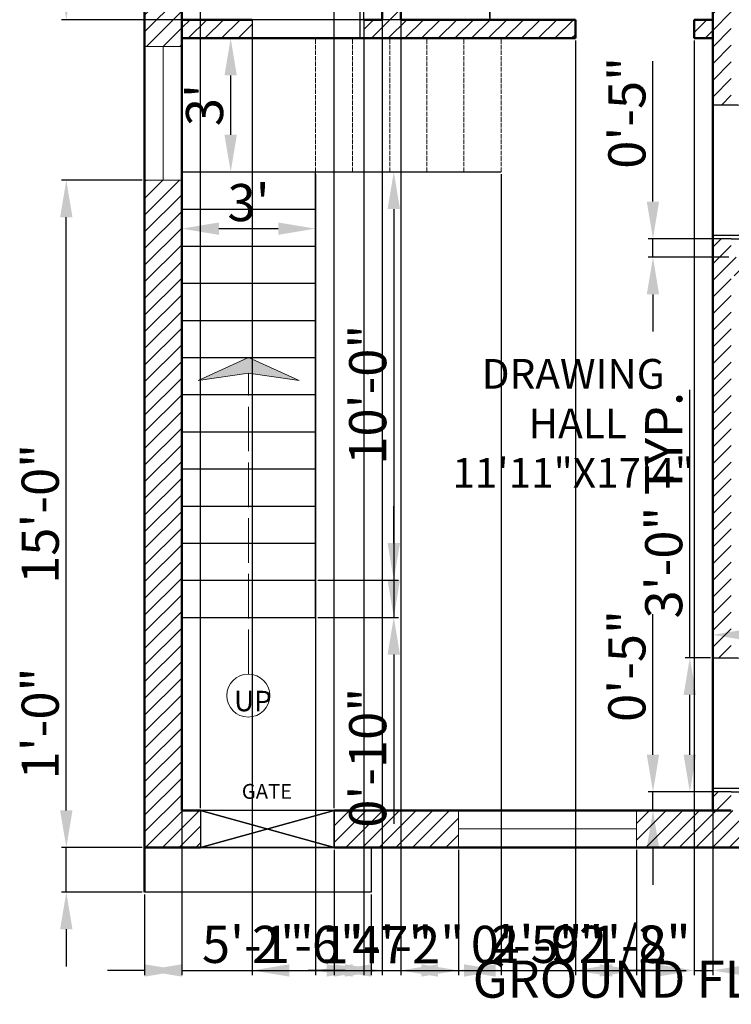
# Model space of a CAD drawing. Units: inches. Extents: x 2305 to 2787, y 1816 to 2216.
# Tile 1 of 3: x 2305 to 2496, y 1816 to 2081. Entities that reach past the tile are written whole.
import ezdxf

# ---------------------------------------------------------------- set-up
doc = ezdxf.new("R2010")
doc.units = ezdxf.units.IN
doc.linetypes.add('ACAD_ISO02W100', pattern=[15, 12, -3])
for name, color, linetype, lineweight in [('A-ANNO-DIMS', 2, 'Continuous', 18), ('A-ANNO-PATH', 253, 'ACAD_ISO02W100', 18), ('A-ANNO-SYMB', 253, 'Continuous', 18), ('A-ANNO-TEXT', 7, 'Continuous', 25), ('A-AREA-IDEN', 7, 'Continuous', 25), ('A-DOOR', 4, 'Continuous', 25), ('A-DOOR-GATE', 240, 'Continuous', 25), ('A-FLOR-FIXT', 8, 'Continuous', 25), ('A-FLOR-STRS', 7, 'Continuous', 25), ('A-FLOR-STRS-OVHD', 253, 'ACAD_ISO02W100', 18), ('A-GLAZ', 4, 'Continuous', 18), ('A-WALL', 7, 'Continuous', 50), ('A-WALL-PATT', 8, 'Continuous', 13)]:
    doc.layers.add(name, color=color, linetype=linetype, lineweight=lineweight)
doc.styles.get("Standard").update_dxf_attribs({"font": 'arial.ttf'})
doc.dimstyles.new('ISO-25', dxfattribs={"dimtxt": 10, "dimasz": 10, "dimexe": 1.25, "dimexo": 0.625, "dimtad": 1, "dimdec": 1, "dimlunit": 3, "dimtxsty": 'Standard', "dimcen": 2.5, "dimadec": 0, "dimazin": 0, "dimtfac": 1, "dimtdec": 1, "dimtmove": 0, "dimatfit": 3, "dimfxl": 1, "dimarcsym": 0})

# ---------------------------------------------------------------- blocks, each defined once
blk = doc.blocks.new('*D7')
at = {"layer": 'A-ANNO-DIMS', "color": 0, "lineweight": -2, "transparency": 16777216}
for p, q in [((2348.79, 2076), (2362.59, 2076)), ((2361.34, 2050), (2361.34, 2066)), ((2348.79, 2040), (2362.59, 2040))]:
    blk.add_line(p, q, dxfattribs=at)
at = {"layer": 'A-ANNO-DIMS', "color": 0, "transparency": 16777216}
for points in [[(2359.67, 2066), (2363, 2066), (2361.34, 2076)], [(2359.67, 2050), (2363, 2050), (2361.34, 2040)]]:
    blk.add_solid(points, dxfattribs=at)
at = {"layer": 'Defpoints', "color": 0, "transparency": 16777216}
for p in [(2348.17, 2076), (2361.34, 2076), (2348.17, 2040)]:
    blk.add_point(p, dxfattribs=at)
at = {"layer": 'A-ANNO-DIMS', "color": 0, "transparency": 16777216, "insert": (2355.6, 2058), "char_height": 10, "attachment_point": 5, "rotation": 90}
blk.add_mtext("3'", dxfattribs=at)
blk = doc.blocks.new('*D8')
at = {"layer": 'A-ANNO-DIMS', "color": 0, "lineweight": -2, "transparency": 16777216}
for p, q in [((2348.17, 2029.37), (2348.17, 2023.46)), ((2384.17, 2029.37), (2384.17, 2023.46)), ((2358.17, 2024.71), (2374.17, 2024.71))]:
    blk.add_line(p, q, dxfattribs=at)
at = {"layer": 'A-ANNO-DIMS', "color": 0, "transparency": 16777216}
for points in [[(2358.17, 2026.37), (2358.17, 2023.04), (2348.17, 2024.71)], [(2374.17, 2026.37), (2374.17, 2023.04), (2384.17, 2024.71)]]:
    blk.add_solid(points, dxfattribs=at)
at = {"layer": 'Defpoints', "color": 0, "transparency": 16777216}
for p in [(2348.17, 2030), (2384.17, 2030), (2384.17, 2024.71)]:
    blk.add_point(p, dxfattribs=at)
at = {"layer": 'A-ANNO-DIMS', "color": 0, "transparency": 16777216, "insert": (2366.17, 2030.44), "char_height": 10, "attachment_point": 5}
blk.add_mtext("3'", dxfattribs=at)
blk = doc.blocks.new('DOOR-SWING-36IN')
for p, q in [((5, 36), (0, 36)), ((0, 1), (41, 1)), ((5, 0), (0, 0)), ((5, 0), (41, 0))]:
    blk.add_line(p, q)
blk.add_arc((5.5, 0.5), 35.5, 359.1931, 90.8069)
blk = doc.blocks.new('WINDOW-36IN')
for p, q in [((0, 10), (0, 0)), ((36, 10), (36, 0)), ((0, 5), (36, 5))]:
    blk.add_line(p, q)
blk = doc.blocks.new('*D18')
at = {"layer": 'A-ANNO-DIMS', "color": 0, "lineweight": -2, "transparency": 16777216}
for p, q in [((2491.17, 1909.76), (2491.17, 1916.55)), ((2501.17, 1915.3), (2522.3, 1915.3)), ((2532.3, 1909.76), (2532.3, 1916.55)), ((2532.3, 1915.3), (2649.8, 1915.3))]:
    blk.add_line(p, q, dxfattribs=at)
at = {"layer": 'A-ANNO-DIMS', "color": 0, "transparency": 16777216}
for points in [[(2501.17, 1916.97), (2501.17, 1913.63), (2491.17, 1915.3)], [(2522.3, 1916.97), (2522.3, 1913.63), (2532.3, 1915.3)]]:
    blk.add_solid(points, dxfattribs=at)
at = {"layer": 'Defpoints', "color": 0, "transparency": 16777216}
for p in [(2532.3, 1915.3), (2491.17, 1909.13), (2532.3, 1909.13)]:
    blk.add_point(p, dxfattribs=at)
at = {"layer": 'A-ANNO-DIMS', "color": 0, "transparency": 16777216, "insert": (2596.05, 1921.1), "char_height": 10, "attachment_point": 5}
blk.add_mtext('DOOR 3\'-5" TYP.', dxfattribs=at)
blk = doc.blocks.new('*D19')
at = {"layer": 'A-ANNO-DIMS', "color": 0, "lineweight": -2, "transparency": 16777216}
for p, q in [((2485, 1909.13), (2485, 1981.33)), ((2490.54, 1909.13), (2483.75, 1909.13)), ((2485, 1883), (2485, 1899.13)), ((2490.54, 1873), (2483.75, 1873))]:
    blk.add_line(p, q, dxfattribs=at)
at = {"layer": 'A-ANNO-DIMS', "color": 0, "transparency": 16777216}
for points in [[(2483.33, 1899.13), (2486.66, 1899.13), (2485, 1909.13)], [(2483.33, 1883), (2486.66, 1883), (2485, 1873)]]:
    blk.add_solid(points, dxfattribs=at)
at = {"layer": 'Defpoints', "color": 0, "transparency": 16777216}
for p in [(2485, 1909.13), (2491.17, 1909.13), (2491.17, 1873)]:
    blk.add_point(p, dxfattribs=at)
at = {"layer": 'A-ANNO-DIMS', "color": 0, "transparency": 16777216, "insert": (2479.26, 1950.23), "char_height": 10, "attachment_point": 5, "rotation": 90}
blk.add_mtext('3\'-0" TYP.', dxfattribs=at)
blk = doc.blocks.new('*D29')
at = {"layer": 'A-ANNO-DIMS', "color": 0, "lineweight": -2, "transparency": 16777216}
for p, q in [((2348.17, 1868.62), (2348.17, 2180.35)), ((2353.17, 1868.62), (2353.17, 2180.35)), ((2338.17, 2179.1), (2328.17, 2179.1)), ((2348.17, 2179.1), (2353.17, 2179.1)), ((2363.17, 2179.1), (2401, 2179.1))]:
    blk.add_line(p, q, dxfattribs=at)
at = {"layer": 'A-ANNO-DIMS', "color": 0, "transparency": 16777216}
for points in [[(2338.17, 2180.76), (2338.17, 2177.43), (2348.17, 2179.1)], [(2363.17, 2180.76), (2363.17, 2177.43), (2353.17, 2179.1)]]:
    blk.add_solid(points, dxfattribs=at)
at = {"layer": 'Defpoints', "color": 0, "transparency": 16777216}
for p in [(2353.17, 2179.1), (2348.17, 1868), (2353.17, 1868)]:
    blk.add_point(p, dxfattribs=at)
at = {"layer": 'A-ANNO-DIMS', "color": 0, "transparency": 16777216, "insert": (2387.08, 2184.83), "char_height": 10, "attachment_point": 5}
blk.add_mtext('0\'-5"', dxfattribs=at)
blk = doc.blocks.new('*D30')
at = {"layer": 'A-ANNO-DIMS', "color": 0, "lineweight": -2, "transparency": 16777216}
for p, q in [((2353.17, 1868.62), (2353.17, 2180.35)), ((2389.17, 1868.62), (2389.17, 2180.35)), ((2363.17, 2179.1), (2379.17, 2179.1))]:
    blk.add_line(p, q, dxfattribs=at)
at = {"layer": 'A-ANNO-DIMS', "color": 0, "transparency": 16777216}
for points in [[(2363.17, 2180.76), (2363.17, 2177.43), (2353.17, 2179.1)], [(2379.17, 2180.76), (2379.17, 2177.43), (2389.17, 2179.1)]]:
    blk.add_solid(points, dxfattribs=at)
at = {"layer": 'Defpoints', "color": 0, "transparency": 16777216}
for p in [(2389.17, 2179.1), (2353.17, 1868), (2389.17, 1868)]:
    blk.add_point(p, dxfattribs=at)
at = {"layer": 'A-ANNO-DIMS', "color": 0, "transparency": 16777216, "insert": (2371.17, 2184.83), "char_height": 10, "attachment_point": 5}
blk.add_mtext('3\'-0"', dxfattribs=at)
blk = doc.blocks.new('*D31')
at = {"layer": 'A-ANNO-DIMS', "color": 0, "lineweight": -2, "transparency": 16777216}
for p, q in [((2389.17, 1857.37), (2389.17, 1823.65)), ((2422.67, 1857.37), (2422.67, 1823.65)), ((2399.17, 1824.9), (2412.67, 1824.9)), ((2422.67, 1824.9), (2483.97, 1824.9))]:
    blk.add_line(p, q, dxfattribs=at)
at = {"layer": 'A-ANNO-DIMS', "color": 0, "transparency": 16777216}
for points in [[(2399.17, 1826.56), (2399.17, 1823.23), (2389.17, 1824.9)], [(2412.67, 1826.56), (2412.67, 1823.23), (2422.67, 1824.9)]]:
    blk.add_solid(points, dxfattribs=at)
at = {"layer": 'Defpoints', "color": 0, "transparency": 16777216}
for p in [(2389.17, 1858), (2422.67, 1858), (2422.67, 1824.9)]:
    blk.add_point(p, dxfattribs=at)
at = {"layer": 'A-ANNO-DIMS', "color": 0, "transparency": 16777216, "insert": (2458.32, 1830.69), "char_height": 10, "attachment_point": 5}
blk.add_mtext('2\'-9 1/2"', dxfattribs=at)
blk = doc.blocks.new('*D32')
at = {"layer": 'A-ANNO-DIMS', "color": 0, "lineweight": -2, "transparency": 16777216}
for p, q in [((2422.67, 1857.37), (2422.67, 1823.65)), ((2470.67, 1857.37), (2470.67, 1823.65)), ((2432.67, 1824.9), (2460.67, 1824.9))]:
    blk.add_line(p, q, dxfattribs=at)
at = {"layer": 'A-ANNO-DIMS', "color": 0, "transparency": 16777216}
for points in [[(2432.67, 1826.56), (2432.67, 1823.23), (2422.67, 1824.9)], [(2460.67, 1826.56), (2460.67, 1823.23), (2470.67, 1824.9)]]:
    blk.add_solid(points, dxfattribs=at)
at = {"layer": 'Defpoints', "color": 0, "transparency": 16777216}
for p in [(2422.67, 1858), (2470.67, 1858), (2470.67, 1824.9)]:
    blk.add_point(p, dxfattribs=at)
at = {"layer": 'A-ANNO-DIMS', "color": 0, "transparency": 16777216, "insert": (2446.67, 1830.63), "char_height": 10, "attachment_point": 5}
blk.add_mtext('4\'-0"', dxfattribs=at)
blk = doc.blocks.new('*D34')
at = {"layer": 'A-ANNO-DIMS', "color": 0, "lineweight": -2, "transparency": 16777216}
for p, q in [((2337.54, 2037.78), (2315.82, 2037.78)), ((2317.07, 1868), (2317.07, 2027.78)), ((2337.54, 1858), (2315.82, 1858))]:
    blk.add_line(p, q, dxfattribs=at)
at = {"layer": 'A-ANNO-DIMS', "color": 0, "transparency": 16777216}
for points in [[(2315.4, 2027.78), (2318.73, 2027.78), (2317.07, 2037.78)], [(2315.4, 1868), (2318.73, 1868), (2317.07, 1858)]]:
    blk.add_solid(points, dxfattribs=at)
at = {"layer": 'Defpoints', "color": 0, "transparency": 16777216}
for p in [(2317.07, 2037.78), (2338.17, 2037.78), (2338.17, 1858)]:
    blk.add_point(p, dxfattribs=at)
at = {"layer": 'A-ANNO-DIMS', "color": 0, "transparency": 16777216, "insert": (2311.34, 1947.89), "char_height": 10, "attachment_point": 5, "rotation": 90}
blk.add_mtext('15\'-0"', dxfattribs=at)
blk = doc.blocks.new('*D35')
at = {"layer": 'A-ANNO-DIMS', "color": 0, "lineweight": -2, "transparency": 16777216}
for p, q in [((2338.17, 1845.37), (2338.17, 1823.65)), ((2399.17, 1845.37), (2399.17, 1823.65)), ((2348.17, 1824.9), (2389.17, 1824.9))]:
    blk.add_line(p, q, dxfattribs=at)
at = {"layer": 'A-ANNO-DIMS', "color": 0, "transparency": 16777216}
for points in [[(2348.17, 1826.56), (2348.17, 1823.23), (2338.17, 1824.9)], [(2389.17, 1826.56), (2389.17, 1823.23), (2399.17, 1824.9)]]:
    blk.add_solid(points, dxfattribs=at)
at = {"layer": 'Defpoints', "color": 0, "transparency": 16777216}
for p in [(2338.17, 1846), (2399.17, 1846), (2399.17, 1824.9)]:
    blk.add_point(p, dxfattribs=at)
at = {"layer": 'A-ANNO-DIMS', "color": 0, "transparency": 16777216, "insert": (2368.67, 1830.63), "char_height": 10, "attachment_point": 5}
blk.add_mtext('5\'-1"', dxfattribs=at)
blk = doc.blocks.new('*D36')
at = {"layer": 'A-ANNO-DIMS', "color": 0, "lineweight": -2, "transparency": 16777216}
for p, q in [((2317.07, 1868), (2317.07, 1904.89)), ((2337.54, 1858), (2315.82, 1858)), ((2317.07, 1846), (2317.07, 1858)), ((2337.54, 1846), (2315.82, 1846)), ((2317.07, 1836), (2317.07, 1826))]:
    blk.add_line(p, q, dxfattribs=at)
at = {"layer": 'A-ANNO-DIMS', "color": 0, "transparency": 16777216}
for points in [[(2315.4, 1868), (2318.73, 1868), (2317.07, 1858)], [(2315.4, 1836), (2318.73, 1836), (2317.07, 1846)]]:
    blk.add_solid(points, dxfattribs=at)
at = {"layer": 'Defpoints', "color": 0, "transparency": 16777216}
for p in [(2317.07, 1858), (2338.17, 1858), (2338.17, 1846)]:
    blk.add_point(p, dxfattribs=at)
at = {"layer": 'A-ANNO-DIMS', "color": 0, "transparency": 16777216, "insert": (2311.34, 1891.44), "char_height": 10, "attachment_point": 5, "rotation": 90}
blk.add_mtext('1\'-0"', dxfattribs=at)
blk = doc.blocks.new('*D37')
at = {"layer": 'A-ANNO-DIMS', "color": 0, "lineweight": -2, "transparency": 16777216}
for p, q in [((2367.17, 2080.37), (2367.17, 1823.65)), ((2397.17, 2080.37), (2397.17, 1823.65)), ((2377.17, 1824.9), (2387.17, 1824.9))]:
    blk.add_line(p, q, dxfattribs=at)
at = {"layer": 'A-ANNO-DIMS', "color": 0, "transparency": 16777216}
for points in [[(2377.17, 1826.56), (2377.17, 1823.23), (2367.17, 1824.9)], [(2387.17, 1826.56), (2387.17, 1823.23), (2397.17, 1824.9)]]:
    blk.add_solid(points, dxfattribs=at)
at = {"layer": 'Defpoints', "color": 0, "transparency": 16777216}
for p in [(2367.17, 2081), (2397.17, 2081), (2397.17, 1824.9)]:
    blk.add_point(p, dxfattribs=at)
at = {"layer": 'A-ANNO-DIMS', "color": 0, "transparency": 16777216, "insert": (2382.17, 1830.63), "char_height": 10, "attachment_point": 5}
blk.add_mtext('2\'-6"', dxfattribs=at)
blk = doc.blocks.new('*D38')
at = {"layer": 'A-ANNO-DIMS', "color": 0, "lineweight": -2, "transparency": 16777216}
for p, q in [((2454.17, 2075.37), (2454.17, 1823.65)), ((2486.17, 2075.37), (2486.17, 1823.65)), ((2464.17, 1824.9), (2476.17, 1824.9))]:
    blk.add_line(p, q, dxfattribs=at)
at = {"layer": 'A-ANNO-DIMS', "color": 0, "transparency": 16777216}
for points in [[(2464.17, 1826.56), (2464.17, 1823.23), (2454.17, 1824.9)], [(2476.17, 1826.56), (2476.17, 1823.23), (2486.17, 1824.9)]]:
    blk.add_solid(points, dxfattribs=at)
at = {"layer": 'Defpoints', "color": 0, "transparency": 16777216}
for p in [(2454.17, 2076), (2486.17, 2076), (2486.17, 1824.9)]:
    blk.add_point(p, dxfattribs=at)
at = {"layer": 'A-ANNO-DIMS', "color": 0, "transparency": 16777216, "insert": (2470.17, 1830.63), "char_height": 10, "attachment_point": 5}
blk.add_mtext('2\'-8"', dxfattribs=at)
blk = doc.blocks.new('*D39')
at = {"layer": 'A-ANNO-DIMS', "color": 0, "lineweight": -2, "transparency": 16777216}
for p, q in [((2402.17, 2147.37), (2402.17, 1823.65)), ((2407.17, 2147.37), (2407.17, 1823.65)), ((2392.17, 1824.9), (2382.17, 1824.9)), ((2402.17, 1824.9), (2407.17, 1824.9)), ((2417.17, 1824.9), (2455, 1824.9))]:
    blk.add_line(p, q, dxfattribs=at)
at = {"layer": 'A-ANNO-DIMS', "color": 0, "transparency": 16777216}
for points in [[(2392.17, 1826.56), (2392.17, 1823.23), (2402.17, 1824.9)], [(2417.17, 1826.56), (2417.17, 1823.23), (2407.17, 1824.9)]]:
    blk.add_solid(points, dxfattribs=at)
at = {"layer": 'Defpoints', "color": 0, "transparency": 16777216}
for p in [(2402.17, 2148), (2407.17, 2148), (2407.17, 1824.9)]:
    blk.add_point(p, dxfattribs=at)
at = {"layer": 'A-ANNO-DIMS', "color": 0, "transparency": 16777216, "insert": (2441.08, 1830.63), "char_height": 10, "attachment_point": 5}
blk.add_mtext('0\'-5"', dxfattribs=at)
blk = doc.blocks.new('*D40')
at = {"layer": 'A-ANNO-DIMS', "color": 0, "lineweight": -2, "transparency": 16777216}
for p, q in [((2384.79, 2040), (2406.52, 2040)), ((2405.27, 2030), (2405.27, 1930)), ((2384.79, 1920), (2406.52, 1920))]:
    blk.add_line(p, q, dxfattribs=at)
at = {"layer": 'A-ANNO-DIMS', "color": 0, "transparency": 16777216}
for points in [[(2403.6, 2030), (2406.93, 2030), (2405.27, 2040)], [(2403.6, 1930), (2406.93, 1930), (2405.27, 1920)]]:
    blk.add_solid(points, dxfattribs=at)
at = {"layer": 'Defpoints', "color": 0, "transparency": 16777216}
for p in [(2384.17, 2040), (2384.17, 1920), (2405.27, 1920)]:
    blk.add_point(p, dxfattribs=at)
at = {"layer": 'A-ANNO-DIMS', "color": 0, "transparency": 16777216, "insert": (2399.54, 1980), "char_height": 10, "attachment_point": 5, "rotation": 90}
blk.add_mtext('10\'-0"', dxfattribs=at)
blk = doc.blocks.new('*D41')
at = {"layer": 'A-ANNO-DIMS', "color": 0, "lineweight": -2, "transparency": 16777216}
for p, q in [((2405.27, 1940), (2405.27, 1950)), ((2384.79, 1930), (2406.52, 1930)), ((2405.27, 1930), (2405.27, 1920)), ((2384.79, 1920), (2406.52, 1920)), ((2405.27, 1910), (2405.27, 1864.39))]:
    blk.add_line(p, q, dxfattribs=at)
at = {"layer": 'A-ANNO-DIMS', "color": 0, "transparency": 16777216}
for points in [[(2403.6, 1940), (2406.93, 1940), (2405.27, 1930)], [(2403.6, 1910), (2406.93, 1910), (2405.27, 1920)]]:
    blk.add_solid(points, dxfattribs=at)
at = {"layer": 'Defpoints', "color": 0, "transparency": 16777216}
for p in [(2384.17, 1930), (2384.17, 1920), (2405.27, 1920)]:
    blk.add_point(p, dxfattribs=at)
at = {"layer": 'A-ANNO-DIMS', "color": 0, "transparency": 16777216, "insert": (2399.54, 1882.19), "char_height": 10, "attachment_point": 5, "rotation": 90}
blk.add_mtext('0\'-10"', dxfattribs=at)
blk = doc.blocks.new('*D42')
at = {"layer": 'A-ANNO-DIMS', "color": 0, "lineweight": -2, "transparency": 16777216}
for p, q in [((2384.17, 2039.37), (2384.17, 1823.65)), ((2434.17, 2039.37), (2434.17, 1823.65)), ((2394.17, 1824.9), (2424.17, 1824.9))]:
    blk.add_line(p, q, dxfattribs=at)
at = {"layer": 'A-ANNO-DIMS', "color": 0, "transparency": 16777216}
for points in [[(2394.17, 1826.56), (2394.17, 1823.23), (2384.17, 1824.9)], [(2424.17, 1826.56), (2424.17, 1823.23), (2434.17, 1824.9)]]:
    blk.add_solid(points, dxfattribs=at)
at = {"layer": 'Defpoints', "color": 0, "transparency": 16777216}
for p in [(2384.17, 2040), (2434.17, 2040), (2434.17, 1824.9)]:
    blk.add_point(p, dxfattribs=at)
at = {"layer": 'A-ANNO-DIMS', "color": 0, "transparency": 16777216, "insert": (2409.17, 1830.54), "char_height": 10, "attachment_point": 5}
blk.add_mtext('4\'-2"', dxfattribs=at)
blk = doc.blocks.new('*D43')
at = {"layer": 'A-ANNO-DIMS', "color": 0, "lineweight": -2, "transparency": 16777216}
for p, q in [((2475.07, 2032), (2475.07, 2069.83)), ((2495.54, 2022), (2473.82, 2022)), ((2475.07, 2017), (2475.07, 2022)), ((2495.54, 2017), (2473.82, 2017)), ((2475.07, 2007), (2475.07, 1997))]:
    blk.add_line(p, q, dxfattribs=at)
at = {"layer": 'A-ANNO-DIMS', "color": 0, "transparency": 16777216}
for points in [[(2473.4, 2032), (2476.73, 2032), (2475.07, 2022)], [(2473.4, 2007), (2476.73, 2007), (2475.07, 2017)]]:
    blk.add_solid(points, dxfattribs=at)
at = {"layer": 'Defpoints', "color": 0, "transparency": 16777216}
for p in [(2475.07, 2022), (2496.17, 2022), (2496.17, 2017)]:
    blk.add_point(p, dxfattribs=at)
at = {"layer": 'A-ANNO-DIMS', "color": 0, "transparency": 16777216, "insert": (2469.34, 2055.91), "char_height": 10, "attachment_point": 5, "rotation": 90}
blk.add_mtext('0\'-5"', dxfattribs=at)
blk = doc.blocks.new('*D44')
at = {"layer": 'A-ANNO-DIMS', "color": 0, "lineweight": -2, "transparency": 16777216}
for p, q in [((2475.07, 1883), (2475.07, 1920.83)), ((2495.54, 1873), (2473.82, 1873)), ((2475.07, 1868), (2475.07, 1873)), ((2495.54, 1868), (2473.82, 1868)), ((2475.07, 1858), (2475.07, 1848))]:
    blk.add_line(p, q, dxfattribs=at)
at = {"layer": 'A-ANNO-DIMS', "color": 0, "transparency": 16777216}
for points in [[(2473.4, 1883), (2476.73, 1883), (2475.07, 1873)], [(2473.4, 1858), (2476.73, 1858), (2475.07, 1868)]]:
    blk.add_solid(points, dxfattribs=at)
at = {"layer": 'Defpoints', "color": 0, "transparency": 16777216}
for p in [(2475.07, 1873), (2496.17, 1873), (2496.17, 1868)]:
    blk.add_point(p, dxfattribs=at)
at = {"layer": 'A-ANNO-DIMS', "color": 0, "transparency": 16777216, "insert": (2469.34, 1906.91), "char_height": 10, "attachment_point": 5, "rotation": 90}
blk.add_mtext('0\'-5"', dxfattribs=at)
blk = doc.blocks.new('*D45')
at = {"layer": 'A-ANNO-DIMS', "color": 0, "lineweight": -2, "transparency": 16777216}
for p, q in [((2486.17, 2075.37), (2486.17, 1823.65)), ((2491.17, 2075.37), (2491.17, 1823.65)), ((2476.17, 1824.9), (2466.17, 1824.9)), ((2486.17, 1824.9), (2491.17, 1824.9)), ((2501.17, 1824.9), (2539, 1824.9))]:
    blk.add_line(p, q, dxfattribs=at)
at = {"layer": 'A-ANNO-DIMS', "color": 0, "transparency": 16777216}
for points in [[(2476.17, 1826.56), (2476.17, 1823.23), (2486.17, 1824.9)], [(2501.17, 1826.56), (2501.17, 1823.23), (2491.17, 1824.9)]]:
    blk.add_solid(points, dxfattribs=at)
at = {"layer": 'Defpoints', "color": 0, "transparency": 16777216}
for p in [(2486.17, 2076), (2491.17, 2076), (2491.17, 1824.9)]:
    blk.add_point(p, dxfattribs=at)
at = {"layer": 'A-ANNO-DIMS', "color": 0, "transparency": 16777216, "insert": (2525.08, 1830.63), "char_height": 10, "attachment_point": 5}
blk.add_mtext('0\'-5"', dxfattribs=at)
blk = doc.blocks.new('*D46')
at = {"layer": 'A-ANNO-DIMS', "color": 0, "lineweight": -2, "transparency": 16777216}
for p, q in [((2348.17, 2080.37), (2348.17, 1823.65)), ((2367.17, 2080.37), (2367.17, 1823.65)), ((2338.17, 1824.9), (2328.17, 1824.9)), ((2348.17, 1824.9), (2367.17, 1824.9)), ((2377.17, 1824.9), (2414.06, 1824.9))]:
    blk.add_line(p, q, dxfattribs=at)
at = {"layer": 'A-ANNO-DIMS', "color": 0, "transparency": 16777216}
for points in [[(2338.17, 1826.56), (2338.17, 1823.23), (2348.17, 1824.9)], [(2377.17, 1826.56), (2377.17, 1823.23), (2367.17, 1824.9)]]:
    blk.add_solid(points, dxfattribs=at)
at = {"layer": 'Defpoints', "color": 0, "transparency": 16777216}
for p in [(2348.17, 2081), (2367.17, 2081), (2367.17, 1824.9)]:
    blk.add_point(p, dxfattribs=at)
at = {"layer": 'A-ANNO-DIMS', "color": 0, "transparency": 16777216, "insert": (2400.61, 1830.54), "char_height": 10, "attachment_point": 5}
blk.add_mtext('1\'-7"', dxfattribs=at)
blk = doc.blocks.new('*D47')
at = {"layer": 'A-ANNO-DIMS', "color": 0, "lineweight": -2, "transparency": 16777216}
for p, q in [((2407.17, 2081.62), (2407.17, 2180.35)), ((2431.17, 2081.62), (2431.17, 2180.35)), ((2417.17, 2179.1), (2421.17, 2179.1)), ((2431.17, 2179.1), (2469.17, 2179.1))]:
    blk.add_line(p, q, dxfattribs=at)
at = {"layer": 'A-ANNO-DIMS', "color": 0, "transparency": 16777216}
for points in [[(2417.17, 2180.76), (2417.17, 2177.43), (2407.17, 2179.1)], [(2421.17, 2180.76), (2421.17, 2177.43), (2431.17, 2179.1)]]:
    blk.add_solid(points, dxfattribs=at)
at = {"layer": 'Defpoints', "color": 0, "transparency": 16777216}
for p in [(2431.17, 2179.1), (2407.17, 2081), (2431.17, 2081)]:
    blk.add_point(p, dxfattribs=at)
at = {"layer": 'A-ANNO-DIMS', "color": 0, "transparency": 16777216, "insert": (2455.17, 2184.83), "char_height": 10, "attachment_point": 5}
blk.add_mtext('2\'-0"', dxfattribs=at)
blk = doc.blocks.new('*D48')
at = {"layer": 'A-ANNO-DIMS', "color": 0, "lineweight": -2, "transparency": 16777216}
for p, q in [((2430.54, 2124), (2315.82, 2124)), ((2317.07, 2114), (2317.07, 2091)), ((2430.54, 2081), (2315.82, 2081))]:
    blk.add_line(p, q, dxfattribs=at)
at = {"layer": 'A-ANNO-DIMS', "color": 0, "transparency": 16777216}
for points in [[(2315.4, 2114), (2318.73, 2114), (2317.07, 2124)], [(2315.4, 2091), (2318.73, 2091), (2317.07, 2081)]]:
    blk.add_solid(points, dxfattribs=at)
at = {"layer": 'Defpoints', "color": 0, "transparency": 16777216}
for p in [(2431.17, 2124), (2317.07, 2081), (2431.17, 2081)]:
    blk.add_point(p, dxfattribs=at)
at = {"layer": 'A-ANNO-DIMS', "color": 0, "transparency": 16777216, "insert": (2311.33, 2102.5), "char_height": 10, "attachment_point": 5, "rotation": 90}
blk.add_mtext('3\'-7"', dxfattribs=at)

msp = doc.modelspace()

# ---------------------------------------------------------------- hatches: boundary and pattern name
at = {"layer": 'A-ANNO-SYMB'}
h = msp.add_hatch(color=256, dxfattribs=at)
h.dxf.hatch_style = 1
h.paths.add_polyline_path([(2366.17, 1990), (2352.58, 1983.77), (2366.17, 1985.81), (2379.76, 1983.77)])
at = {"layer": 'A-WALL-PATT'}
h = msp.add_hatch(dxfattribs=at)
h.set_pattern_fill('ANSI31', color=256)
h.paths.add_polyline_path([(2435.17, 2158), (2387.17, 2158), (2387.17, 2148), (2402.17, 2148), (2402.17, 2081), (2397.17, 2081), (2397.17, 2076), (2402.17, 2076), (2454.17, 2076), (2454.17, 2081), (2407.17, 2081), (2407.17, 2148), (2435.17, 2148)])
h.paths.add_polyline_path([(2363.17, 2158), (2338.17, 2158), (2338.17, 2073.78), (2348.17, 2073.78), (2348.17, 2076), (2348.17, 2148), (2363.17, 2148)])
h.paths.add_polyline_path([(2544.17, 2158), (2463.17, 2158), (2463.17, 2148), (2496.17, 2148), (2544.17, 2148)])
h.paths.add_polyline_path([(2496.17, 2148), (2491.17, 2148), (2491.17, 2081), (2491.17, 2058), (2496.17, 2058)])
h.paths.add_polyline_path([(2638.17, 2158), (2580.17, 2158), (2580.17, 2148), (2628.17, 2148), (2628.17, 2108.13), (2628.28, 2108.13), (2628.25, 2048.13), (2628.17, 2012), (2628.17, 1970), (2628.28, 1970), (2628.25, 1910), (2628.17, 1868), (2580.17, 1868), (2580.17, 1858), (2638.17, 1858)])
h.paths.add_polyline_path([(2628.17, 2017), (2496.17, 2017), (2496.17, 2022), (2491.17, 2022), (2491.17, 1909), (2496.17, 1909), (2496.17, 2012), (2628.17, 2012)])
h.paths.add_polyline_path([(2544.17, 1868), (2496.17, 1868), (2470.67, 1868), (2470.67, 1858), (2544.17, 1858)])
h.paths.add_polyline_path([(2422.67, 1868), (2402.17, 1868), (2389.17, 1868), (2389.17, 1858), (2422.67, 1858)])
h.paths.add_polyline_path([(2353.17, 1868), (2348.17, 1868), (2348.17, 2037.78), (2338.17, 2037.78), (2338.17, 1858), (2353.17, 1858)])
h = msp.add_hatch(dxfattribs=at)
h.set_pattern_fill('ANSI31', color=256)
h.paths.add_polyline_path([(2367.17, 2081), (2348.17, 2081), (2348.17, 2076), (2367.17, 2076)])
h = msp.add_hatch(dxfattribs=at)
h.set_pattern_fill('ANSI31', color=256)
h.paths.add_polyline_path([(2496.17, 1873), (2491.17, 1873), (2491.17, 1868), (2496.17, 1868)])
h.paths.add_polyline_path([(2491.17, 2081), (2486.17, 2081), (2486.17, 2076), (2491.17, 2076)])

# ---------------------------------------------------------------- linework, layer by layer
at = {"layer": 'A-ANNO-PATH'}
msp.add_line((2366.17, 1904.73), (2366.17, 1985.81), dxfattribs=at)
at = {"layer": 'A-ANNO-SYMB'}
for p, q in [((2366.17, 1990), (2352.58, 1983.77)), ((2366.17, 1990), (2379.76, 1983.77)), ((2352.58, 1983.77), (2366.17, 1985.81)), ((2379.76, 1983.77), (2366.17, 1985.81))]:
    msp.add_line(p, q, dxfattribs=at)
msp.add_circle((2366.09, 1898.94), 5.78, dxfattribs=at)
at = {"layer": 'A-DOOR'}
for p, q in [((2396.17, 2076), (2396.17, 2111)), ((2397.17, 2081), (2397.17, 2111)), ((2367.17, 2081), (2367.17, 2076)), ((2397.17, 2081), (2397.17, 2076))]:
    msp.add_line(p, q, dxfattribs=at)
at = {"layer": 'A-DOOR-GATE'}
for p, q in [((2353.17, 1868), (2353.17, 1858)), ((2353.17, 1858), (2389.17, 1868)), ((2389.17, 1858), (2353.17, 1868)), ((2389.17, 1868), (2353.17, 1868)), ((2353.17, 1868), (2353.17, 1858)), ((2389.17, 1868), (2353.17, 1868)), ((2353.17, 1868), (2389.17, 1858)), ((2389.17, 1868), (2353.17, 1858)), ((2389.17, 1868), (2389.17, 1858)), ((2389.17, 1858), (2389.17, 1868)), ((2389.17, 1858), (2389.17, 1868)), ((2389.17, 1858), (2353.17, 1858)), ((2353.17, 1858), (2389.17, 1858))]:
    msp.add_line(p, q, dxfattribs=at)
at = {"layer": 'A-FLOR-FIXT'}
msp.add_line((2431.17, 2124), (2431.17, 2081), dxfattribs=at)
at = {"layer": 'A-FLOR-STRS'}
for p, q in [((2348.17, 2040), (2384.17, 2040)), ((2384.17, 1920), (2384.17, 2040)), ((2384.17, 2040), (2434.17, 2040)), ((2348.17, 2030), (2384.17, 2030)), ((2348.17, 2020), (2384.17, 2020)), ((2348.17, 2010), (2384.17, 2010)), ((2348.17, 2000), (2384.17, 2000)), ((2348.17, 1990), (2384.17, 1990)), ((2348.17, 1980), (2384.17, 1980)), ((2348.17, 1970), (2384.17, 1970)), ((2348.17, 1960), (2384.17, 1960)), ((2348.17, 1950), (2384.17, 1950)), ((2348.17, 1940), (2384.17, 1940)), ((2348.17, 1930), (2384.17, 1930)), ((2348.17, 1920), (2384.17, 1920)), ((2389.17, 1858), (2399.17, 1858)), ((2399.17, 1858), (2399.17, 1846)), ((2399.17, 1846), (2338.17, 1846))]:
    msp.add_line(p, q, dxfattribs=at)
at = {"layer": 'A-FLOR-STRS-OVHD', "ltscale": 0.1}
for p, q in [((2384.17, 2040), (2384.17, 2076)), ((2394.17, 2040), (2394.17, 2076)), ((2404.17, 2040), (2404.17, 2076)), ((2414.17, 2040), (2414.17, 2076)), ((2424.17, 2040), (2424.17, 2076)), ((2434.17, 2040), (2434.17, 2076))]:
    msp.add_line(p, q, dxfattribs=at)
at = {"layer": 'A-GLAZ'}
for p, q in [((2422.67, 1868), (2422.67, 1858)), ((2470.67, 1868), (2470.67, 1858)), ((2422.67, 1863), (2470.67, 1863))]:
    msp.add_line(p, q, dxfattribs=at)
at = {"layer": 'A-WALL'}
for p, q in [((2338.17, 1846), (2338.17, 2158)), ((2348.17, 2076), (2348.17, 2148)), ((2402.17, 2148), (2402.17, 2081)), ((2407.17, 2148), (2407.17, 2081)), ((2491.17, 2148), (2491.17, 2081)), ((2348.17, 2081), (2367.17, 2081)), ((2397.17, 2081), (2402.17, 2081)), ((2407.17, 2081), (2454.17, 2081)), ((2454.17, 2081), (2454.17, 2076)), ((2486.17, 2081), (2486.17, 2076)), ((2486.17, 2081), (2491.17, 2081)), ((2491.17, 2081), (2491.17, 1868)), ((2348.17, 1868), (2348.17, 2076)), ((2348.17, 2076), (2402.17, 2076)), ((2402.17, 2076), (2454.17, 2076)), ((2486.17, 2076), (2491.17, 2076)), ((2353.17, 1868), (2348.17, 1868)), ((2402.17, 1868), (2389.17, 1868)), ((2496.17, 1868), (2402.17, 1868)), ((2353.17, 1858), (2338.17, 1858)), ((2638.17, 1858), (2389.17, 1858))]:
    msp.add_line(p, q, dxfattribs=at)

# ---------------------------------------------------------------- block references
at = {"layer": 'A-DOOR'}
for p in [(2491.17, 2022), (2491.17, 1873)]:
    msp.add_blockref('DOOR-SWING-36IN', p, dxfattribs=at)
at = {"layer": 'A-GLAZ', "rotation": 89.99999999999896}
msp.add_blockref('WINDOW-36IN', (2348.17, 2037.78), dxfattribs=at)

# ---------------------------------------------------------------- texts
at = {"layer": 'A-ANNO-TEXT', "attachment_point": 1}
for s, width, insert, char_height in [('UP', 17.3956, (2362.24, 1900.22), 5.5), ('GATE', 26.8923, (2364.33, 1875.13), 4), ('{\\fArial|b1|i0|c0|p34;GROUND FLOOR PLAN}', 215.2333, (2426.52, 1827.56), 10)]:
    msp.add_mtext_dynamic_manual_height_columns(s, width=width, gutter_width=12.5, heights=[0], dxfattribs=dict(at, insert=insert, char_height=char_height))
at = {"layer": 'A-AREA-IDEN', "insert": (2400.63, 1989.6), "char_height": 8, "attachment_point": 1}
msp.add_mtext_dynamic_manual_height_columns('\\pxqc;DRAWING\\P HALL\\P11\'11"X17\'4"', width=105.9041, gutter_width=12.5, heights=[0], dxfattribs=at)

# ---------------------------------------------------------------- dimensions: what is measured, and where the dimension line sits
at = {"layer": 'A-ANNO-DIMS'}
for base, p1, p2, override, picture, middle in [((2353.17, 2179.1), (2348.17, 1868), (2353.17, 1868), {"dimdec": 1, "dimlfac": 1, "dimrnd": 0, "dimzin": 1, "dimdsep": 46, "dimlunit": 4, "dimfrac": 2}, '*D29', (2387.08, 2184.83)), ((2389.17, 2179.1), (2353.17, 1868), (2389.17, 1868), {"dimdec": 1, "dimlfac": 1, "dimrnd": 0, "dimzin": 1, "dimdsep": 46, "dimlunit": 4, "dimfrac": 2}, '*D30', (2371.17, 2184.83)), ((2431.17, 2179.1), (2407.17, 2081), (2431.17, 2081), {"dimdec": 1, "dimlfac": 1, "dimrnd": 0, "dimzin": 1, "dimdsep": 46, "dimlunit": 4, "dimfrac": 2}, '*D47', (2455.17, 2184.83)), ((2407.17, 1824.9), (2402.17, 2148), (2407.17, 2148), {"dimdec": 1, "dimlfac": 1, "dimrnd": 0, "dimzin": 1, "dimdsep": 46, "dimlunit": 4, "dimfrac": 2}, '*D39', (2441.08, 1830.63)), ((2367.17, 1824.9), (2348.17, 2081), (2367.17, 2081), {"dimdec": 1, "dimlfac": 1, "dimrnd": 0, "dimzin": 1, "dimdsep": 46, "dimlunit": 4, "dimfrac": 2}, '*D46', (2400.61, 1830.54)), ((2397.17, 1824.9), (2367.17, 2081), (2397.17, 2081), {"dimdec": 1, "dimlfac": 1, "dimrnd": 0, "dimzin": 1, "dimdsep": 46, "dimlunit": 4, "dimfrac": 2}, '*D37', (2382.17, 1830.63)), ((2486.17, 1824.9), (2454.17, 2076), (2486.17, 2076), {"dimdec": 1, "dimlfac": 1, "dimrnd": 0, "dimzin": 1, "dimdsep": 46, "dimlunit": 4, "dimfrac": 2}, '*D38', (2470.17, 1830.63)), ((2491.17, 1824.9), (2486.17, 2076), (2491.17, 2076), {"dimdec": 1, "dimlfac": 1, "dimrnd": 0, "dimzin": 1, "dimdsep": 46, "dimlunit": 4, "dimfrac": 2}, '*D45', (2525.08, 1830.63)), ((2434.17, 1824.9), (2384.17, 2040), (2434.17, 2040), {"dimdec": 1, "dimlfac": 1, "dimrnd": 0, "dimzin": 1, "dimdsep": 46, "dimlunit": 4, "dimfrac": 2}, '*D42', (2409.17, 1830.54)), ((2384.17, 2024.71), (2348.17, 2030), (2384.17, 2030), {"dimclrd": 0, "dimclre": 0, "dimclrt": 0}, '*D8', (2366.17, 2030.44)), ((2422.67, 1824.9), (2389.17, 1858), (2422.67, 1858), {"dimdec": 1, "dimlfac": 1, "dimrnd": 0, "dimzin": 1, "dimdsep": 46, "dimlunit": 4, "dimfrac": 2}, '*D31', (2458.32, 1830.69)), ((2470.67, 1824.9), (2422.67, 1858), (2470.67, 1858), {"dimdec": 1, "dimlfac": 1, "dimrnd": 0, "dimzin": 1, "dimdsep": 46, "dimlunit": 4, "dimfrac": 2}, '*D32', (2446.67, 1830.63)), ((2399.17, 1824.9), (2338.17, 1846), (2399.17, 1846), {"dimdec": 1, "dimlfac": 1, "dimrnd": 0, "dimzin": 1, "dimdsep": 46, "dimlunit": 4, "dimfrac": 2}, '*D35', (2368.67, 1830.63))]:
    dim = msp.add_linear_dim(base=base, p1=p1, p2=p2, dimstyle='ISO-25', override=override, dxfattribs=at)
    dim.commit()
    dim.dimension.update_dxf_attribs({"geometry": picture, "text_midpoint": middle})
for base, p1, p2, angle, override, picture, middle in [((2317.07, 2081), (2431.17, 2124), (2431.17, 2081), 90, {"dimdec": 1, "dimlfac": 1, "dimrnd": 0, "dimzin": 1, "dimdsep": 46, "dimlunit": 4, "dimfrac": 2}, '*D48', (2311.33, 2102.5)), ((2361.34, 2076), (2348.17, 2040), (2348.17, 2076), 90, {"dimclrd": 0, "dimclre": 0, "dimclrt": 0}, '*D7', (2355.6, 2058)), ((2475.07, 2022), (2496.17, 2017), (2496.17, 2022), 90, {"dimdec": 1, "dimlfac": 1, "dimrnd": 0, "dimzin": 1, "dimdsep": 46, "dimlunit": 4, "dimfrac": 2}, '*D43', (2469.34, 2055.91)), ((2405.27, 1920), (2384.17, 2040), (2384.17, 1920), 270, {"dimdec": 1, "dimlfac": 1, "dimrnd": 0, "dimzin": 1, "dimdsep": 46, "dimlunit": 4, "dimfrac": 2}, '*D40', (2399.54, 1980)), ((2317.07, 2037.78), (2338.17, 1858), (2338.17, 2037.78), 90, {"dimdec": 1, "dimlfac": 1, "dimrnd": 0, "dimzin": 1, "dimdsep": 46, "dimlunit": 4, "dimfrac": 2}, '*D34', (2311.34, 1947.89)), ((2405.27, 1920), (2384.17, 1930), (2384.17, 1920), 270, {"dimdec": 1, "dimlfac": 1, "dimrnd": 0, "dimzin": 1, "dimdsep": 46, "dimlunit": 4, "dimfrac": 2}, '*D41', (2399.54, 1882.19)), ((2475.07, 1873), (2496.17, 1868), (2496.17, 1873), 90, {"dimdec": 1, "dimlfac": 1, "dimrnd": 0, "dimzin": 1, "dimdsep": 46, "dimlunit": 4, "dimfrac": 2}, '*D44', (2469.34, 1906.91)), ((2317.07, 1858), (2338.17, 1846), (2338.17, 1858), 90, {"dimdec": 1, "dimlfac": 1, "dimrnd": 0, "dimzin": 1, "dimdsep": 46, "dimlunit": 4, "dimfrac": 2}, '*D36', (2311.34, 1891.44))]:
    dim = msp.add_linear_dim(base=base, p1=p1, p2=p2, angle=angle, dimstyle='ISO-25', override=override, dxfattribs=at)
    dim.commit()
    dim.dimension.update_dxf_attribs({"geometry": picture, "text_midpoint": middle})
dim = msp.add_linear_dim(base=(2485, 1909.13), p1=(2491.17, 1873), p2=(2491.17, 1909.13), angle=90, text='<> TYP.', dimstyle='ISO-25', override={"dimdec": 1, "dimlfac": 1, "dimrnd": 0, "dimzin": 1, "dimdsep": 46, "dimlunit": 4, "dimfrac": 2}, dxfattribs=at)
dim.commit()
dim.dimension.update_dxf_attribs({"geometry": '*D19', "text_midpoint": (2479.26, 1950.23)})
dim = msp.add_linear_dim(base=(2532.3, 1915.3), p1=(2491.17, 1909.13), p2=(2532.3, 1909.13), text='DOOR <> TYP.', dimstyle='ISO-25', override={"dimdec": 1, "dimlfac": 1, "dimrnd": 0, "dimzin": 1, "dimdsep": 46, "dimlunit": 4, "dimfrac": 2}, dxfattribs=at)
dim.commit()
dim.dimension.update_dxf_attribs({"geometry": '*D18', "text_midpoint": (2596.05, 1921.1)})

doc.saveas('drawing.dxf')
